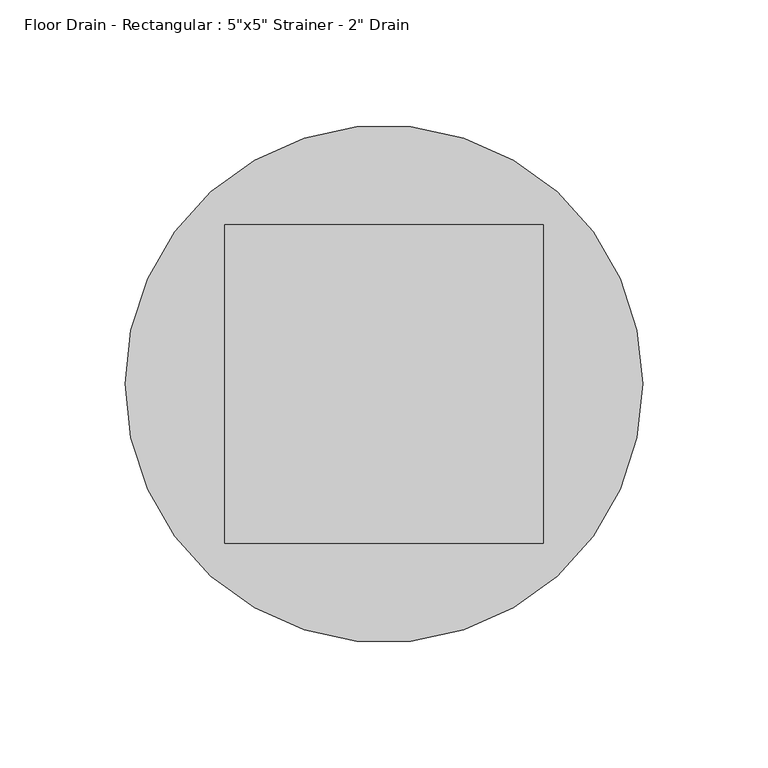
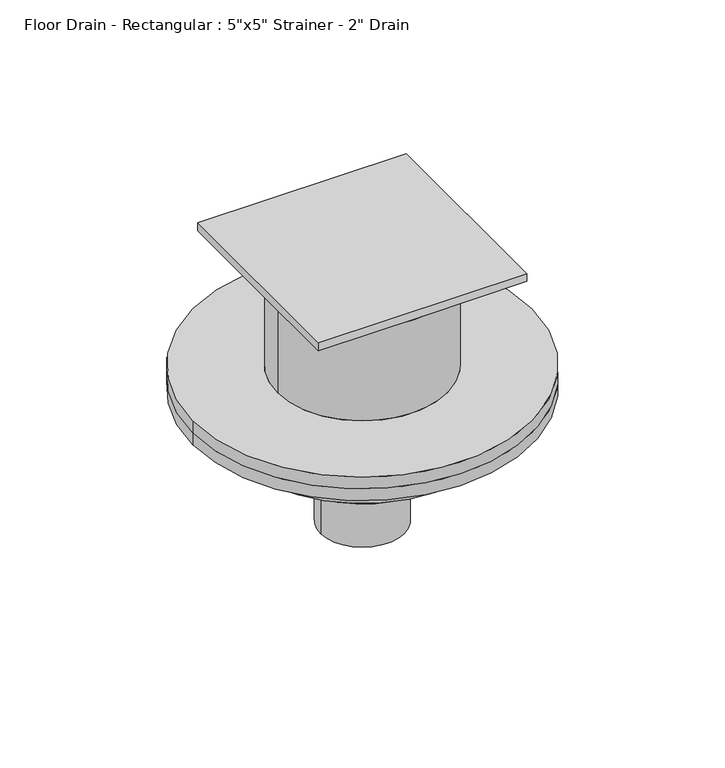
"""IFC4 building model written with IfcOpenShell, lengths in millimetres: flow terminal geometry."""

from ifc_helpers import new_model, si_unit, frame, origin, place, context, project, spatial, polyline, circle_curve, source, transform, mapped, element, save
from ifc_brep_helpers import plane_surface, cylinder_surface, revolved_surface, advanced_brep


def flow_terminal_2b63360b(model_context):
    return source(origin(), model_context, "Body", "AdvancedBrep", [
        advanced_brep(
        [(103.1875, 0.0, -74.93), (-103.1875, 0.0, -74.93), (-51.59375, 0.0, -74.93), (51.59375, 0.0, -74.93), (103.1875, 0.0, -82.55), (-103.1875, 0.0, -82.55), (51.59375, 0.0, -15.24), (-51.59375, 0.0, -15.24), (-63.5, 0.0, -5.08), (0.0, 63.5, -5.08), (63.5, 0.0, -5.08), (0.0, -63.5, -5.08), (63.5, 63.5, 0.0), (-63.5, 63.5, 0.0), (-63.5, -63.5, 0.0), (63.5, -63.5, 0.0), (-63.5, -63.5, -5.08), (-63.5, 63.5, -5.08), (63.5, 63.5, -5.08), (63.5, -63.5, -5.08)],
        [
            (0, 1, circle_curve(frame((0.0, 0.0, -74.93), z_axis=(0.0, 0.0, 1.0), x_axis=(-1.0, 0.0, 0.0)), 103.1875)),
            (1, 0, circle_curve(frame((0.0, 0.0, -74.93), z_axis=(0.0, 0.0, 1.0), x_axis=(-1.0, 0.0, 0.0)), 103.1875)),
            (2, 3, circle_curve(frame((0.0, 0.0, -74.93), z_axis=(0.0, 0.0, -1.0), x_axis=(-1.0, 0.0, 0.0)), 51.59375)),
            (3, 2, circle_curve(frame((0.0, 0.0, -74.93), z_axis=(0.0, 0.0, -1.0), x_axis=(-1.0, 0.0, 0.0)), 51.59375)),
            (4, 5, circle_curve(frame((0.0, 0.0, -82.55), z_axis=(0.0, 0.0, -1.0), x_axis=(-1.0, 0.0, 0.0)), 103.1875)),
            (5, 4, circle_curve(frame((0.0, 0.0, -82.55), z_axis=(0.0, 0.0, -1.0), x_axis=(-1.0, 0.0, 0.0)), 103.1875)),
            (0, 4),
            (5, 1),
            (6, 3),
            (2, 7),
            (7, 6, circle_curve(frame((0.0, 0.0, -15.24), z_axis=(0.0, 0.0, -1.0), x_axis=(-1.0, 0.0, 0.0)), 51.59375)),
            (6, 7, circle_curve(frame((0.0, 0.0, -15.24), z_axis=(0.0, 0.0, -1.0), x_axis=(-1.0, 0.0, 0.0)), 51.59375)),
            (7, 8),
            (8, 9, circle_curve(frame((0.0, 0.0, -5.08), z_axis=(0.0, 0.0, -1.0), x_axis=(-1.0, 0.0, 0.0)), 63.5)),
            (9, 10, circle_curve(frame((0.0, 0.0, -5.08), z_axis=(0.0, 0.0, -1.0), x_axis=(-1.0, 0.0, 0.0)), 63.5)),
            (10, 6),
            (10, 11, circle_curve(frame((0.0, 0.0, -5.08), z_axis=(0.0, 0.0, -1.0), x_axis=(-1.0, 0.0, 0.0)), 63.5)),
            (11, 8, circle_curve(frame((0.0, 0.0, -5.08), z_axis=(0.0, 0.0, -1.0), x_axis=(-1.0, 0.0, 0.0)), 63.5)),
            (12, 13),
            (13, 14),
            (14, 15),
            (15, 12),
            (16, 8),
            (11, 16),
            (8, 17),
            (17, 9),
            (18, 10),
            (9, 18),
            (10, 19),
            (19, 11),
            (12, 18),
            (17, 13),
            (16, 14),
            (19, 15),
        ],
        [
            plane_surface(frame((-103.1875, 0.0, -74.93), z_axis=(0.0, 0.0, 1.0), x_axis=(0.0, -1.0, 0.0))),
            plane_surface(frame((-103.1875, 0.0, -82.55), z_axis=(0.0, 0.0, -1.0), x_axis=(0.0, 1.0, 0.0))),
            cylinder_surface(frame((0.0, 0.0, -82.55), z_axis=(0.0, 0.0, 1.0), x_axis=(-1.0, 0.0, 0.0)), 103.1875),
            cylinder_surface(frame((0.0, 0.0, -74.93), z_axis=(0.0, 0.0, 1.0), x_axis=(-1.0, 0.0, 0.0)), 51.59375),
            revolved_surface(polyline([(-63.5, 0.0, -5.08), (-51.59375, 0.0, -15.24)]), (0.0, 0.0, -5.08), (0.0, 0.0, -1.0)),
            plane_surface(frame((-63.5, 63.5, 0.0), z_axis=(0.0, 0.0, 1.0), x_axis=(-1.0, 0.0, 0.0))),
            plane_surface(frame((-63.5, 63.5, -5.08), z_axis=(0.0, 0.0, -1.0), x_axis=(1.0, 0.0, 0.0))),
            plane_surface(frame((63.5, 63.5, 0.0), z_axis=(0.0, 1.0, 0.0), x_axis=(0.0, 0.0, -1.0))),
            plane_surface(frame((-63.5, 63.5, 0.0), z_axis=(-1.0, 0.0, 0.0), x_axis=(0.0, 0.0, -1.0))),
            plane_surface(frame((-63.5, -63.5, 0.0), z_axis=(0.0, -1.0, 0.0), x_axis=(0.0, 0.0, -1.0))),
            plane_surface(frame((63.5, -63.5, 0.0), z_axis=(1.0, 0.0, 0.0), x_axis=(0.0, 0.0, -1.0))),
        ],
        [
            (0, [[1, 2], [3, 4]]),
            (1, [[5, 6]]),
            (2, [[-1, 7, -6, 8]]),
            (2, [[-2, -8, -5, -7]]),
            (3, [[9, -3, 10, 11]]),
            (3, [[-9, 12, -10, -4]]),
            (4, [[13, 14, 15, 16, -11]]),
            (4, [[-13, -12, -16, 17, 18]]),
            (5, [[19, 20, 21, 22]]),
            (6, [[23, -18, 24]]),
            (6, [[25, 26, -14]]),
            (6, [[27, -15, 28]]),
            (6, [[29, 30, -17]]),
            (7, [[-19, 31, -28, -26, 32]]),
            (8, [[-20, -32, -25, -23, 33]]),
            (9, [[-21, -33, -24, -30, 34]]),
            (10, [[-22, -34, -29, -27, -31]]),
        ],
    ),
        advanced_brep(
        [(103.1875, 0.0, -82.55), (-103.1875, 0.0, -82.55), (103.1875, 0.0, -90.17), (-103.1875, 0.0, -90.17), (77.2583333, 0.0, -90.17), (-77.2583333, 0.0, -90.17), (77.2583333, 0.0, -110.1725), (-77.2583333, 0.0, -110.1725), (51.3291667, 0.0, -110.1725), (-51.3291667, 0.0, -110.1725), (25.4, 0.0, -174.625), (-25.4, 0.0, -174.625), (-25.4, 0.0, -128.5875), (25.4, 0.0, -128.5875), (51.3291667, 0.0, -128.5875), (-51.3291667, 0.0, -128.5875)],
        [
            (0, 1, circle_curve(frame((0.0, 0.0, -82.55), z_axis=(0.0, 0.0, 1.0), x_axis=(-1.0, 0.0, 0.0)), 103.1875)),
            (1, 0, circle_curve(frame((0.0, 0.0, -82.55), z_axis=(0.0, 0.0, 1.0), x_axis=(-1.0, 0.0, 0.0)), 103.1875)),
            (2, 3, circle_curve(frame((0.0, 0.0, -90.17), z_axis=(0.0, 0.0, -1.0), x_axis=(-1.0, 0.0, 0.0)), 103.1875)),
            (3, 2, circle_curve(frame((0.0, 0.0, -90.17), z_axis=(0.0, 0.0, -1.0), x_axis=(-1.0, 0.0, 0.0)), 103.1875)),
            (4, 5, circle_curve(frame((0.0, 0.0, -90.17), z_axis=(0.0, 0.0, 1.0), x_axis=(-1.0, 0.0, 0.0)), 77.2583333)),
            (5, 4, circle_curve(frame((0.0, 0.0, -90.17), z_axis=(0.0, 0.0, 1.0), x_axis=(-1.0, 0.0, 0.0)), 77.2583333)),
            (0, 2),
            (3, 1),
            (6, 7, circle_curve(frame((0.0, 0.0, -110.1725), z_axis=(0.0, 0.0, -1.0), x_axis=(-1.0, 0.0, 0.0)), 77.2583333)),
            (7, 6, circle_curve(frame((0.0, 0.0, -110.1725), z_axis=(0.0, 0.0, -1.0), x_axis=(-1.0, 0.0, 0.0)), 77.2583333)),
            (8, 9, circle_curve(frame((0.0, 0.0, -110.1725), z_axis=(0.0, 0.0, 1.0), x_axis=(-1.0, 0.0, 0.0)), 51.3291667)),
            (9, 8, circle_curve(frame((0.0, 0.0, -110.1725), z_axis=(0.0, 0.0, 1.0), x_axis=(-1.0, 0.0, 0.0)), 51.3291667)),
            (7, 5),
            (4, 6),
            (10, 11, circle_curve(frame((0.0, 0.0, -174.625), z_axis=(0.0, 0.0, -1.0), x_axis=(-1.0, 0.0, 0.0)), 25.4)),
            (11, 10, circle_curve(frame((0.0, 0.0, -174.625), z_axis=(0.0, 0.0, -1.0), x_axis=(-1.0, 0.0, 0.0)), 25.4)),
            (11, 12),
            (12, 13, circle_curve(frame((0.0, 0.0, -128.5875), z_axis=(0.0, 0.0, -1.0), x_axis=(-1.0, 0.0, 0.0)), 25.4)),
            (13, 10),
            (13, 12, circle_curve(frame((0.0, 0.0, -128.5875), z_axis=(0.0, 0.0, -1.0), x_axis=(-1.0, 0.0, 0.0)), 25.4)),
            (14, 15, circle_curve(frame((0.0, 0.0, -128.5875), z_axis=(0.0, 0.0, -1.0), x_axis=(-1.0, 0.0, 0.0)), 51.3291667)),
            (15, 14, circle_curve(frame((0.0, 0.0, -128.5875), z_axis=(0.0, 0.0, -1.0), x_axis=(-1.0, 0.0, 0.0)), 51.3291667)),
            (15, 9),
            (8, 14),
        ],
        [
            plane_surface(frame((-103.1875, 0.0, -82.55), z_axis=(0.0, 0.0, 1.0), x_axis=(0.0, -1.0, 0.0))),
            plane_surface(frame((-103.1875, 0.0, -90.17), z_axis=(0.0, 0.0, -1.0), x_axis=(0.0, 1.0, 0.0))),
            cylinder_surface(frame((0.0, 0.0, -90.17), z_axis=(0.0, 0.0, 1.0), x_axis=(-1.0, 0.0, 0.0)), 103.1875),
            plane_surface(frame((-77.2583333, 0.0, -110.1725), z_axis=(0.0, 0.0, -1.0), x_axis=(0.0, 1.0, 0.0))),
            cylinder_surface(frame((0.0, 0.0, -110.1725), z_axis=(0.0, 0.0, 1.0), x_axis=(-1.0, 0.0, 0.0)), 77.2583333),
            plane_surface(frame((-25.4, 0.0, -174.625), z_axis=(0.0, 0.0, -1.0), x_axis=(0.0, 1.0, 0.0))),
            cylinder_surface(frame((0.0, 0.0, -174.625), z_axis=(0.0, 0.0, 1.0), x_axis=(-1.0, 0.0, 0.0)), 25.4),
            plane_surface(frame((-51.3291667, 0.0, -128.5875), z_axis=(0.0, 0.0, -1.0), x_axis=(0.0, 1.0, 0.0))),
            cylinder_surface(frame((0.0, 0.0, -128.5875), z_axis=(0.0, 0.0, 1.0), x_axis=(-1.0, 0.0, 0.0)), 51.3291667),
        ],
        [
            (0, [[1, 2]]),
            (1, [[3, 4], [5, 6]]),
            (2, [[-1, 7, -4, 8]]),
            (2, [[-2, -8, -3, -7]]),
            (3, [[9, 10], [11, 12]]),
            (4, [[-10, 13, -5, 14]]),
            (4, [[-9, -14, -6, -13]]),
            (5, [[15, 16]]),
            (6, [[-16, 17, 18, 19]]),
            (6, [[-15, -19, 20, -17]]),
            (7, [[21, 22], [-18, -20]]),
            (8, [[-22, 23, -11, 24]]),
            (8, [[-21, -24, -12, -23]]),
        ],
    ),
    ])


if __name__ == "__main__":
    model = new_model("IFC4")
    model_context = context("Model", 3, world=origin())
    ifc_project = project(units=[si_unit("LENGTHUNIT", "METRE", prefix="MILLI")], contexts=[model_context])
    site = spatial("IfcSite", under=ifc_project)
    building = spatial("IfcBuilding", under=site)
    placement = place(None, origin())
    flow_terminal_shape = flow_terminal_2b63360b(model_context)
    element("IfcFlowTerminal", 1, ObjectType="Floor Drain - Rectangular : 5\"x5\" Strainer - 2\" Drain", at=placement, inside=building, context=model_context, shape_type="MappedRepresentation", body=[
        mapped(flow_terminal_shape, transform((0.0, 0.0, 0.0), x_axis=(1.0, 0.0, 0.0), y_axis=(0.0, 1.0, 0.0), z_axis=(0.0, 0.0, 1.0))),
    ])
    save(model, "model.ifc")

# Revit data of these elements
# Type "Floor Drain - Rectangular : 5\"x5\" Strainer - 2\" Drain"
#   WFU = 2
#   Strainer Height = 0' - 3 1/4"
#   Half Strainer Length = 0' - 2 1/2"
#   Strainer Length = 0' - 5"
#   Radius 2 = 0' - 3.04167"
#   Radius 1 = 0' - 2.02083"
#   Radius 3 = 0' - 2 1/32"
#   Pipe Radius = 1"
#   Pipe Diameter = 2"
#   Height 2 = 0' - 0.725"
#   Height 1 = 0' - 1 13/16"
#   Body Radius = 0' - 4 1/16"
#   Body Height = 0' - 3 5/8"
#   Body Diameter = 0' - 8 1/8"
#   Drain Material = none
#   HWFU = 0
#   Default Elevation = 0
#   CWFU = 0
